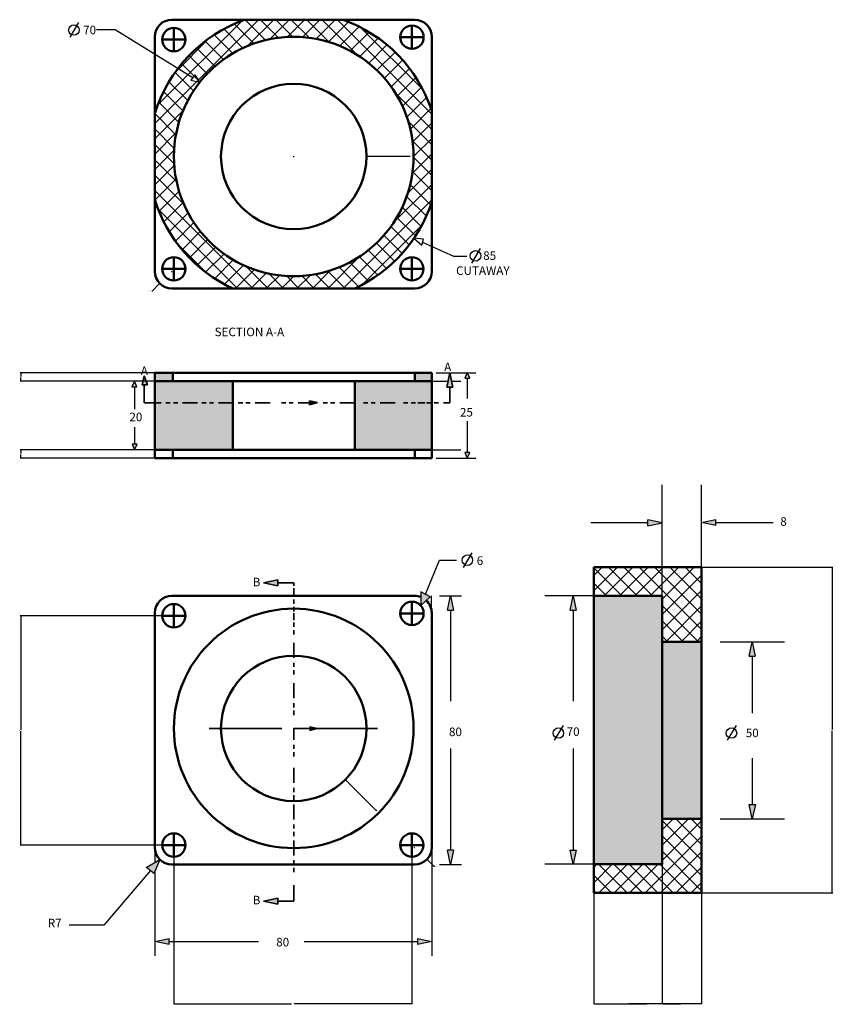
# Model space of a CAD drawing. Units: millimetres. Extents: x 2682 to 5504, y 1503 to 3069.
# Tile 1 of 1: x 2682.4 to 2920.1, y 1503.5 to 1791.3. Entities that reach past the tile are written whole.
import ezdxf

# ---------------------------------------------------------------- set-up
doc = ezdxf.new("R2010")
doc.units = ezdxf.units.MM
doc.linetypes.add('PHANTOM', pattern=[63.5, 31.75, -6.35, 6.35, -6.35, 6.35, -6.35])
for name, color, linetype, lineweight in [('M-DIMS', 2, 'Continuous', 25), ('M-HATC', 8, 'Continuous', 18), ('M-OUTL', 7, 'Continuous', 50), ('M-SECT', 1, 'PHANTOM', 35), ('M-TEXT', 7, 'Continuous', 25)]:
    doc.layers.add(name, color=color, linetype=linetype, lineweight=lineweight)
doc.styles.get("Standard").update_dxf_attribs({"font": 'arial.ttf'})
doc.dimstyles.get("Standard").update_dxf_attribs({"dimtxt": 0.18, "dimasz": 0.18, "dimexe": 0.18, "dimexo": 0.0625, "dimgap": 0.09, "dimtad": 0, "dimtih": 1, "dimtoh": 1, "dimdec": 4, "dimzin": 0, "dimdsep": 46, "dimtxsty": 'Standard', "dimcen": 0.09, "dimadec": 0, "dimazin": 0, "dimtfac": 1, "dimtdec": 4, "dimtofl": 0, "dimtmove": 0, "dimatfit": 3, "dimfxl": 1, "dimtolj": 1, "dimtzin": 0, "dimarcsym": 0})

# ---------------------------------------------------------------- blocks, each defined once
blk = doc.blocks.new('HOLE-6')
for p, q in [((2727.41, 1721.83), (2727.41, 1715)), ((2724, 1718.42), (2730.82, 1718.42))]:
    blk.add_line(p, q)
blk.add_circle((2727.41, 1718.42), 3.41)
blk = doc.blocks.new('*D2')
at = {"layer": 'Defpoints', "color": 0, "transparency": 16777216}
for p in [(2727.41, 1550.02), (2796.97, 1550.02), (2796.97, 1503.64)]:
    blk.add_point(p, dxfattribs=at)
at = {"layer": 'M-DIMS', "color": 0, "lineweight": -2, "transparency": 16777216}
for p, q in [((2727.41, 1549.96), (2727.41, 1503.46)), ((2796.97, 1549.96), (2796.97, 1503.46)), ((2727.59, 1503.64), (2761.79, 1503.64)), ((2796.79, 1503.64), (2762.58, 1503.64))]:
    blk.add_line(p, q, dxfattribs=at)
at = {"layer": 'M-DIMS', "color": 0, "transparency": 16777216}
for points in [[(2727.59, 1503.67), (2727.59, 1503.61), (2727.41, 1503.64)], [(2796.79, 1503.67), (2796.79, 1503.61), (2796.97, 1503.64)]]:
    blk.add_solid(points, dxfattribs=at)
at = {"layer": 'M-DIMS', "color": 0, "transparency": 16777216, "insert": (2762.19, 1503.64), "char_height": 0.18, "attachment_point": 5}
blk.add_mtext('\\A1;69.56', dxfattribs=at)
blk = doc.blocks.new('*D3')
at = {"layer": 'Defpoints', "color": 0, "transparency": 16777216}
for p in [(2682.68, 1617.03), (2727.41, 1617.03), (2727.41, 1550.02)]:
    blk.add_point(p, dxfattribs=at)
at = {"layer": 'M-DIMS', "color": 0, "lineweight": -2, "transparency": 16777216}
for p, q in [((2727.35, 1617.03), (2682.5, 1617.03)), ((2682.68, 1616.85), (2682.68, 1583.71)), ((2682.68, 1550.2), (2682.68, 1583.34)), ((2727.35, 1550.02), (2682.5, 1550.02))]:
    blk.add_line(p, q, dxfattribs=at)
at = {"layer": 'M-DIMS', "color": 0, "transparency": 16777216}
for points in [[(2682.65, 1616.85), (2682.71, 1616.85), (2682.68, 1617.03)], [(2682.65, 1550.2), (2682.71, 1550.2), (2682.68, 1550.02)]]:
    blk.add_solid(points, dxfattribs=at)
at = {"layer": 'M-DIMS', "color": 0, "transparency": 16777216, "insert": (2682.68, 1583.52), "char_height": 0.18, "attachment_point": 5}
blk.add_mtext('\\A1;67.01', dxfattribs=at)
blk = doc.blocks.new('*D4')
at = {"layer": 'Defpoints', "color": 0, "transparency": 16777216}
for p in [(2850.11, 1544.38), (2870.11, 1544.38), (2870.11, 1503.64)]:
    blk.add_point(p, dxfattribs=at)
at = {"layer": 'M-DIMS', "color": 0, "lineweight": -2, "transparency": 16777216}
for p, q in [((2850.11, 1544.32), (2850.11, 1503.46)), ((2870.11, 1544.32), (2870.11, 1503.46)), ((2850.29, 1503.64), (2859.89, 1503.64)), ((2869.93, 1503.64), (2860.33, 1503.64))]:
    blk.add_line(p, q, dxfattribs=at)
at = {"layer": 'M-DIMS', "color": 0, "transparency": 16777216}
for points in [[(2850.29, 1503.67), (2850.29, 1503.61), (2850.11, 1503.64)], [(2869.93, 1503.67), (2869.93, 1503.61), (2870.11, 1503.64)]]:
    blk.add_solid(points, dxfattribs=at)
at = {"layer": 'M-DIMS', "color": 0, "transparency": 16777216, "insert": (2860.11, 1503.64), "char_height": 0.18, "attachment_point": 5}
blk.add_mtext('\\A1;20', dxfattribs=at)
blk = doc.blocks.new('*D5')
at = {"layer": 'Defpoints', "color": 0, "transparency": 16777216}
for p in [(2850.11, 1536.01), (2881.63, 1536.01), (2881.63, 1503.64)]:
    blk.add_point(p, dxfattribs=at)
at = {"layer": 'M-DIMS', "color": 0, "lineweight": -2, "transparency": 16777216}
for p, q in [((2850.11, 1535.95), (2850.11, 1503.46)), ((2881.63, 1535.95), (2881.63, 1503.46)), ((2850.29, 1503.64), (2865.48, 1503.64)), ((2881.45, 1503.64), (2866.26, 1503.64))]:
    blk.add_line(p, q, dxfattribs=at)
at = {"layer": 'M-DIMS', "color": 0, "transparency": 16777216}
for points in [[(2850.29, 1503.67), (2850.29, 1503.61), (2850.11, 1503.64)], [(2881.45, 1503.67), (2881.45, 1503.61), (2881.63, 1503.64)]]:
    blk.add_solid(points, dxfattribs=at)
at = {"layer": 'M-DIMS', "color": 0, "transparency": 16777216, "insert": (2865.87, 1503.64), "char_height": 0.18, "attachment_point": 5}
blk.add_mtext('\\A1;31.52', dxfattribs=at)
blk = doc.blocks.new('*D6')
at = {"layer": 'Defpoints', "color": 0, "transparency": 16777216}
for p in [(2881.63, 1631.23), (2919.79, 1631.23), (2881.63, 1536.01)]:
    blk.add_point(p, dxfattribs=at)
at = {"layer": 'M-DIMS', "color": 0, "lineweight": -2, "transparency": 16777216}
for p, q in [((2881.69, 1631.23), (2919.97, 1631.23)), ((2919.79, 1631.05), (2919.79, 1583.8)), ((2919.79, 1536.19), (2919.79, 1583.44)), ((2881.69, 1536.01), (2919.97, 1536.01))]:
    blk.add_line(p, q, dxfattribs=at)
at = {"layer": 'M-DIMS', "color": 0, "transparency": 16777216}
for points in [[(2919.76, 1631.05), (2919.82, 1631.05), (2919.79, 1631.23)], [(2919.76, 1536.19), (2919.82, 1536.19), (2919.79, 1536.01)]]:
    blk.add_solid(points, dxfattribs=at)
at = {"layer": 'M-DIMS', "color": 0, "transparency": 16777216, "insert": (2919.79, 1583.62), "char_height": 0.18, "attachment_point": 5}
blk.add_mtext('\\A1;95.22', dxfattribs=at)
blk = doc.blocks.new('*D7')
at = {"layer": 'Defpoints', "color": 0, "transparency": 16777216}
for p in [(2721.84, 1688.06), (2682.68, 1685.56), (2721.84, 1685.56)]:
    blk.add_point(p, dxfattribs=at)
at = {"layer": 'M-DIMS', "color": 0, "lineweight": -2, "transparency": 16777216}
for p, q in [((2721.77, 1688.06), (2682.5, 1688.06)), ((2682.68, 1687.88), (2682.68, 1686.99)), ((2682.68, 1685.74), (2682.68, 1686.63)), ((2721.77, 1685.56), (2682.5, 1685.56))]:
    blk.add_line(p, q, dxfattribs=at)
at = {"layer": 'M-DIMS', "color": 0, "transparency": 16777216}
for points in [[(2682.65, 1687.88), (2682.71, 1687.88), (2682.68, 1688.06)], [(2682.65, 1685.74), (2682.71, 1685.74), (2682.68, 1685.56)]]:
    blk.add_solid(points, dxfattribs=at)
at = {"layer": 'M-DIMS', "color": 0, "transparency": 16777216, "insert": (2682.68, 1686.81), "char_height": 0.18, "attachment_point": 5}
blk.add_mtext('\\A1;2.5', dxfattribs=at)
blk = doc.blocks.new('*D8')
at = {"layer": 'Defpoints', "color": 0, "transparency": 16777216}
for p in [(2747.38, 1599.11), (2777.49, 1569.11)]:
    blk.add_point(p, dxfattribs=at)
at = {"layer": 'M-DIMS', "color": 0, "lineweight": -2, "transparency": 16777216}
for p, q in [((2762.35, 1584.11), (2762.53, 1584.11)), ((2762.44, 1584.02), (2762.44, 1584.2)), ((2786.52, 1560.11), (2777.62, 1568.98)), ((2786.7, 1560.11), (2786.52, 1560.11))]:
    blk.add_line(p, q, dxfattribs=at)
at = {"layer": 'M-DIMS', "color": 0, "transparency": 16777216}
blk.add_solid([(2777.64, 1569), (2777.6, 1568.96), (2777.49, 1569.11)], dxfattribs=at)
at = {"layer": 'M-DIMS', "color": 0, "transparency": 16777216, "insert": (2787.12, 1560.11), "char_height": 0.18, "attachment_point": 5}
blk.add_mtext('\\A1;∅42.5', dxfattribs=at)
blk = doc.blocks.new('*D9')
at = {"layer": 'Defpoints', "color": 0, "transparency": 16777216}
for p in [(2881.63, 1631.23), (2870.11, 1609.4), (2881.63, 1503.64)]:
    blk.add_point(p, dxfattribs=at)
at = {"layer": 'M-DIMS', "color": 0, "lineweight": -2, "transparency": 16777216}
for p, q in [((2881.63, 1631.17), (2881.63, 1503.46)), ((2870.11, 1609.34), (2870.11, 1503.46)), ((2870.29, 1503.64), (2875.49, 1503.64)), ((2881.45, 1503.64), (2876.25, 1503.64))]:
    blk.add_line(p, q, dxfattribs=at)
at = {"layer": 'M-DIMS', "color": 0, "transparency": 16777216}
for points in [[(2870.29, 1503.67), (2870.29, 1503.61), (2870.11, 1503.64)], [(2881.45, 1503.67), (2881.45, 1503.61), (2881.63, 1503.64)]]:
    blk.add_solid(points, dxfattribs=at)
at = {"layer": 'M-DIMS', "color": 0, "transparency": 16777216, "insert": (2875.87, 1503.64), "char_height": 0.18, "attachment_point": 5}
blk.add_mtext('\\A1;11.52', dxfattribs=at)
blk = doc.blocks.new('*D10')
at = {"layer": 'Defpoints', "color": 0, "transparency": 16777216}
for p in [(2721.84, 1665.56), (2682.68, 1663.06), (2721.84, 1663.06)]:
    blk.add_point(p, dxfattribs=at)
at = {"layer": 'M-DIMS', "color": 0, "lineweight": -2, "transparency": 16777216}
for p, q in [((2721.77, 1665.56), (2682.5, 1665.56)), ((2682.68, 1665.38), (2682.68, 1664.49)), ((2682.68, 1663.24), (2682.68, 1664.13)), ((2721.77, 1663.06), (2682.5, 1663.06))]:
    blk.add_line(p, q, dxfattribs=at)
at = {"layer": 'M-DIMS', "color": 0, "transparency": 16777216}
for points in [[(2682.65, 1665.38), (2682.71, 1665.38), (2682.68, 1665.56)], [(2682.65, 1663.24), (2682.71, 1663.24), (2682.68, 1663.06)]]:
    blk.add_solid(points, dxfattribs=at)
at = {"layer": 'M-DIMS', "color": 0, "transparency": 16777216, "insert": (2682.68, 1664.31), "char_height": 0.18, "attachment_point": 5}
blk.add_mtext('\\A1;2.50', dxfattribs=at)
blk = doc.blocks.new('*D11')
at = {"layer": 'Defpoints', "color": 0, "transparency": 16777216}
for p in [(2726.84, 1717.7), (2723.3, 1714.16)]:
    blk.add_point(p, dxfattribs=at)
at = {"layer": 'M-DIMS', "color": 0, "lineweight": -2, "transparency": 16777216}
for p, q in [((2726.75, 1717.7), (2726.93, 1717.7)), ((2726.84, 1717.61), (2726.84, 1717.79)), ((2721.18, 1712.04), (2723.17, 1714.04)), ((2721, 1712.04), (2721.18, 1712.04))]:
    blk.add_line(p, q, dxfattribs=at)
at = {"layer": 'M-DIMS', "color": 0, "transparency": 16777216}
blk.add_solid([(2723.15, 1714.06), (2723.19, 1714.01), (2723.3, 1714.16)], dxfattribs=at)
at = {"layer": 'M-DIMS', "color": 0, "transparency": 16777216, "insert": (2720.39, 1712.04), "char_height": 0.18, "attachment_point": 5}
blk.add_mtext('\\A1;4X R5.00', dxfattribs=at)
blk = doc.blocks.new('*D12')
at = {"layer": 'Defpoints', "color": 0, "transparency": 16777216}
for p in [(2797.77, 1549.3), (2801.36, 1545.82)]:
    blk.add_point(p, dxfattribs=at)
at = {"layer": 'M-DIMS', "color": 0, "lineweight": -2, "transparency": 16777216}
for p, q in [((2797.68, 1549.3), (2797.86, 1549.3)), ((2797.77, 1549.21), (2797.77, 1549.39)), ((2803.52, 1543.73), (2801.49, 1545.7)), ((2803.7, 1543.73), (2803.52, 1543.73))]:
    blk.add_line(p, q, dxfattribs=at)
at = {"layer": 'M-DIMS', "color": 0, "transparency": 16777216}
blk.add_solid([(2801.52, 1545.72), (2801.47, 1545.67), (2801.36, 1545.82)], dxfattribs=at)
at = {"layer": 'M-DIMS', "color": 0, "transparency": 16777216, "insert": (2804.31, 1543.73), "char_height": 0.18, "attachment_point": 5}
blk.add_mtext('\\A1;4X R5.00', dxfattribs=at)
blk = doc.blocks.new('*D13')
at = {"layer": 'Defpoints', "color": 0, "transparency": 16777216}
for p in [(2741.19, 1751.28), (2783.69, 1751.28)]:
    blk.add_point(p, dxfattribs=at)
at = {"layer": 'M-DIMS', "color": 0, "lineweight": -2, "transparency": 16777216}
for p, q in [((2762.35, 1751.28), (2762.53, 1751.28)), ((2762.44, 1751.19), (2762.44, 1751.37)), ((2796.44, 1751.28), (2783.87, 1751.28))]:
    blk.add_line(p, q, dxfattribs=at)
at = {"layer": 'M-DIMS', "color": 0, "transparency": 16777216}
blk.add_solid([(2783.87, 1751.31), (2783.87, 1751.25), (2783.69, 1751.28)], dxfattribs=at)
at = {"layer": 'M-DIMS', "color": 0, "transparency": 16777216, "insert": (2796.93, 1751.28), "char_height": 0.18, "attachment_point": 5}
blk.add_mtext('\\A1;∅42.50', dxfattribs=at)

msp = doc.modelspace()

# ---------------------------------------------------------------- hatches: boundary and pattern name
at = {"layer": 'M-DIMS'}
h = msp.add_hatch(color=256, dxfattribs=at)
h.dxf.hatch_style = 1
h.paths.add_polyline_path([(2715.954, 1685.563), (2715.185, 1683.9), (2716.643, 1683.9)])
h.paths.add_polyline_path([(2718.77, 1687.184), (2718.139, 1684.573), (2719.674, 1684.573)])
h.paths.add_polyline_path([(2716.723, 1667.225), (2715.264, 1667.225), (2715.954, 1665.563)])
h.paths.add_polyline_path([(2813.896, 1664.741), (2812.437, 1664.741), (2813.127, 1663.078)])
h.paths.add_polyline_path([(2813.184, 1688.063), (2813.148, 1688.063), (2812.398, 1686.441), (2813.857, 1686.441)])
h.paths.add_polyline_path([(2808.083, 1688.063), (2807.195, 1683.887), (2808.962, 1683.887)])
h = msp.add_hatch(color=256, dxfattribs=at)
h.dxf.hatch_style = 1
h.paths.add_polyline_path([(2865.934, 1645.043), (2865.934, 1643.277), (2870.11, 1644.165)])
h.paths.add_polyline_path([(2885.806, 1645.132), (2881.63, 1644.253), (2885.806, 1643.365)])
h.paths.add_polyline_path([(2844.062, 1622.82), (2843.174, 1618.644), (2844.94, 1618.644)])
h.paths.add_polyline_path([(2896.438, 1609.402), (2895.55, 1605.226), (2897.316, 1605.226)])
h.paths.add_polyline_path([(2844.95, 1548.557), (2843.184, 1548.557), (2844.062, 1544.381)])
h.paths.add_polyline_path([(2897.326, 1561.875), (2895.56, 1561.875), (2896.438, 1557.699)])
h = msp.add_hatch(color=256, dxfattribs=at)
h.dxf.hatch_style = 1
h.paths.add_polyline_path([(2757.796, 1534.519), (2753.62, 1533.641), (2757.796, 1532.753)])
h.paths.add_polyline_path([(2757.796, 1627.506), (2753.62, 1626.628), (2757.796, 1625.74)])
h = msp.add_hatch(color=256, dxfattribs=at)
h.dxf.hatch_style = 1
h.paths.add_polyline_path([(2799.554, 1624.01), (2799.554, 1620.003, -0.0017904), (2799.57, 1619.984), (2802.295, 1622.604)])
h = msp.add_hatch(color=256, dxfattribs=at)
h.dxf.hatch_style = 1
h.paths.add_polyline_path([(2808.251, 1622.82), (2807.363, 1618.644), (2809.129, 1618.644)])
h.paths.add_polyline_path([(2809.139, 1548.474), (2807.373, 1548.474), (2808.251, 1544.298)])
h.paths.add_polyline_path([(2802.772, 1521.845), (2798.596, 1522.733), (2798.596, 1520.967)])
h.paths.add_polyline_path([(2726.014, 1522.719), (2721.837, 1521.845), (2726.012, 1520.952)])
h.paths.add_polyline_path([(2723.301, 1545.762), (2719.332, 1543.416), (2720.212, 1542.815), (2721.671, 1541.819)])
at = {"layer": 'M-HATC'}
h = msp.add_hatch(dxfattribs=at)
h.set_pattern_fill('ANSI37', color=256)
h.paths.add_polyline_path([(2776.856, 1791.259), (2748.017, 1791.259, 0.2353251), (2721.837, 1763.846), (2721.837, 1738.714, 0.212581), (2744.612, 1712.698), (2780.261, 1712.698, 0.2072631), (2802.772, 1737.889), (2802.772, 1764.671, 0.229956)])
h.paths.add_polyline_path([(2797.436, 1751.28, -1), (2727.436, 1751.28, -1)], flags=16)
h.paths.add_polyline_path([(2783.686, 1751.28, -1), (2741.186, 1751.28, -1)], flags=0)
h = msp.add_hatch(color=256, dxfattribs=at)
h.dxf.hatch_style = 1
h.set_gradient(color1=(69, 84, 165))
h.paths.add_polyline_path([(2727.092, 1688.063), (2721.837, 1688.063), (2721.837, 1685.563), (2727.092, 1685.563)])
h = msp.add_hatch(color=256, dxfattribs=at)
h.dxf.hatch_style = 1
h.set_gradient(color1=(255, 255, 255), color2=(69, 84, 165))
h.paths.add_polyline_path([(2802.772, 1688.063), (2797.847, 1688.063), (2797.847, 1685.563), (2802.772, 1685.563)])
h.paths.add_polyline_path([(2802.772, 1685.563), (2797.847, 1685.563), (2780.261, 1685.563), (2780.261, 1665.563), (2802.772, 1665.563)])
h = msp.add_hatch(color=256, dxfattribs=at)
h.dxf.hatch_style = 1
h.set_gradient(color1=(69, 84, 165))
h.paths.add_polyline_path([(2744.612, 1685.563), (2721.837, 1685.563), (2721.837, 1665.563), (2744.612, 1665.563)])
h = msp.add_hatch(dxfattribs=at)
h.set_pattern_fill('ANSI37', color=256)
h.paths.add_polyline_path([(2881.63, 1631.232), (2850.11, 1631.232), (2850.11, 1622.859), (2870.11, 1622.859), (2870.11, 1609.402), (2881.63, 1609.402)])
h.paths.add_polyline_path([(2881.63, 1557.699), (2870.11, 1557.699), (2870.11, 1544.381), (2850.11, 1544.381), (2850.11, 1536.011), (2881.63, 1536.011)])
h = msp.add_hatch(color=256, dxfattribs=at)
h.dxf.hatch_style = 1
h.set_gradient(color1=(69, 84, 165))
h.paths.add_polyline_path([(2870.11, 1544.381), (2870.11, 1622.859), (2850.11, 1622.859), (2850.11, 1544.381)])
h.paths.add_polyline_path([(2881.63, 1557.699), (2881.63, 1609.402), (2870.11, 1609.402), (2870.11, 1557.699)])
at = {"layer": 'M-SECT'}
h = msp.add_hatch(color=256, dxfattribs=at)
h.dxf.hatch_style = 1
h.paths.add_polyline_path([(2769.415, 1679.384), (2767.094, 1679.869), (2767.094, 1678.731)])
h = msp.add_hatch(color=256, dxfattribs=at)
h.dxf.hatch_style = 1
h.paths.add_polyline_path([(2769.415, 1584.104), (2767.094, 1584.589), (2767.094, 1583.451)])

# ---------------------------------------------------------------- linework, layer by layer
at = {"layer": 'M-DIMS'}
for p, q in [((2699.559, 1790.403), (2696.997, 1786.118)), ((2710.286, 1788.25), (2704.783, 1788.25)), ((2732.939, 1774.293), (2710.286, 1788.25)), ((2733.619, 1775.152), (2732.38, 1773.587)), ((2732.38, 1773.587), (2735.006, 1773.019)), ((2735.006, 1773.019), (2733.619, 1775.152)), ((2797.567, 1727.361), (2799.86, 1725.306)), ((2800.365, 1727.13), (2797.567, 1727.361)), ((2799.86, 1725.306), (2800.365, 1727.13)), ((2800.111, 1726.211), (2809.089, 1722.152)), ((2816.899, 1724.402), (2814.337, 1720.116)), ((2809.089, 1722.152), (2813.032, 1722.152)), ((2804.1, 1688.063), (2815.663, 1688.063)), ((2813.167, 1688.104), (2812.398, 1686.441)), ((2813.857, 1686.441), (2813.167, 1688.104)), ((2718.378, 1685.563), (2710.071, 1685.563)), ((2715.954, 1685.563), (2715.185, 1683.9)), ((2715.185, 1683.9), (2716.643, 1683.9)), ((2716.643, 1683.9), (2715.954, 1685.563)), ((2715.954, 1683.9), (2715.954, 1677.378)), ((2721.837, 1685.563), (2719.331, 1685.563)), ((2802.772, 1685.563), (2807.552, 1685.563)), ((2808.609, 1685.563), (2811.272, 1685.563)), ((2812.398, 1686.441), (2813.857, 1686.441)), ((2813.167, 1686.441), (2813.167, 1680.511)), ((2715.954, 1672.162), (2715.954, 1667.225)), ((2813.167, 1673.937), (2813.167, 1664.741)), ((2716.723, 1667.225), (2715.264, 1667.225)), ((2715.264, 1667.225), (2715.954, 1665.563)), ((2715.954, 1665.563), (2716.723, 1667.225)), ((2721.837, 1665.563), (2710.071, 1665.563)), ((2802.772, 1665.563), (2811.272, 1665.563)), ((2813.896, 1664.741), (2812.437, 1664.741)), ((2812.437, 1664.741), (2813.127, 1663.078)), ((2813.127, 1663.078), (2813.896, 1664.741)), ((2804.1, 1663.063), (2815.663, 1663.063)), ((2813.167, 1663.164), (2813.167, 1663.063)), ((2870.11, 1622.859), (2870.11, 1655.326)), ((2881.63, 1631.232), (2881.63, 1655.326)), ((2865.934, 1644.165), (2849.244, 1644.165)), ((2865.934, 1643.277), (2865.934, 1645.043)), ((2870.11, 1644.165), (2865.934, 1645.043)), ((2865.934, 1643.277), (2865.934, 1645.043)), ((2870.11, 1644.165), (2865.934, 1645.043)), ((2865.934, 1643.277), (2870.11, 1644.165)), ((2865.934, 1643.277), (2870.11, 1644.165)), ((2881.63, 1644.253), (2885.806, 1645.132)), ((2881.63, 1644.253), (2885.806, 1645.132)), ((2885.806, 1643.365), (2881.63, 1644.253)), ((2885.806, 1643.365), (2881.63, 1644.253)), ((2885.806, 1643.365), (2885.806, 1645.132)), ((2885.806, 1643.365), (2885.806, 1645.132)), ((2885.806, 1644.253), (2902.496, 1644.253)), ((2814.529, 1635.453), (2811.967, 1631.167)), ((2800.934, 1623.302), (2805.048, 1633.31)), ((2805.048, 1633.31), (2810.002, 1633.31)), ((2802.295, 1622.604), (2799.554, 1624.01)), ((2799.554, 1624.01), (2799.554, 1620.003)), ((2799.57, 1619.984), (2802.295, 1622.604)), ((2802.666, 1618.881), (2802.666, 1622.82)), ((2805.048, 1622.82), (2811.453, 1622.82)), ((2807.363, 1618.644), (2808.251, 1622.82)), ((2808.251, 1622.82), (2809.129, 1618.644)), ((2850.11, 1622.859), (2835.789, 1622.859)), ((2835.789, 1622.859), (2835.789, 1622.859)), ((2843.174, 1618.644), (2844.062, 1622.82)), ((2844.062, 1622.82), (2844.94, 1618.644)), ((2807.363, 1618.644), (2809.129, 1618.644)), ((2808.251, 1618.644), (2808.251, 1592.071)), ((2843.174, 1618.644), (2844.94, 1618.644)), ((2844.062, 1618.644), (2844.062, 1592.071)), ((2887.083, 1609.402), (2905.793, 1609.402)), ((2895.55, 1605.226), (2896.438, 1609.402)), ((2895.55, 1605.226), (2896.438, 1609.402)), ((2896.438, 1609.402), (2897.316, 1605.226)), ((2896.438, 1609.402), (2897.316, 1605.226)), ((2895.55, 1605.226), (2897.316, 1605.226)), ((2895.55, 1605.226), (2897.316, 1605.226)), ((2896.438, 1605.226), (2896.438, 1588.536)), ((2841.122, 1584.915), (2838.559, 1580.63)), ((2891.685, 1584.915), (2889.123, 1580.63)), ((2808.251, 1578.22), (2808.251, 1548.474)), ((2844.062, 1578.22), (2844.062, 1548.557)), ((2896.438, 1575.406), (2896.438, 1561.875)), ((2896.438, 1557.699), (2895.56, 1561.875)), ((2895.56, 1561.875), (2897.326, 1561.875)), ((2897.326, 1561.875), (2896.438, 1557.699)), ((2887.083, 1557.699), (2905.793, 1557.699)), ((2721.837, 1549.298), (2721.837, 1544.897)), ((2802.772, 1549.298), (2802.772, 1517.637)), ((2809.139, 1548.474), (2807.373, 1548.474)), ((2808.251, 1544.298), (2807.373, 1548.474)), ((2809.139, 1548.474), (2808.251, 1544.298)), ((2844.062, 1544.381), (2843.184, 1548.557)), ((2843.184, 1548.557), (2844.95, 1548.557)), ((2844.95, 1548.557), (2844.062, 1544.381)), ((2719.332, 1543.416), (2723.301, 1545.762)), ((2723.301, 1545.762), (2721.671, 1541.819)), ((2720.212, 1542.815), (2719.332, 1543.416)), ((2720.212, 1542.815), (2721.671, 1541.819)), ((2805.048, 1544.298), (2811.453, 1544.298)), ((2850.11, 1544.381), (2835.789, 1544.381)), ((2720.579, 1542.564), (2706.963, 1526.564)), ((2721.837, 1542.221), (2721.837, 1517.637)), ((2706.963, 1526.564), (2696.837, 1526.564)), ((2721.837, 1521.845), (2726.014, 1522.719)), ((2726.012, 1520.952), (2726.014, 1522.719)), ((2798.596, 1522.733), (2798.596, 1520.967)), ((2798.596, 1522.733), (2802.772, 1521.845)), ((2726.012, 1520.952), (2721.837, 1521.845)), ((2726.013, 1521.845), (2752.192, 1521.845)), ((2765.468, 1521.845), (2798.596, 1521.845)), ((2802.772, 1521.845), (2798.596, 1520.967))]:
    msp.add_line(p, q, dxfattribs=at)
for centre in [(2698.214, 1788.229), (2815.554, 1722.227), (2813.184, 1633.278), (2839.776, 1582.741), (2890.34, 1582.741)]:
    msp.add_circle(centre, 1.535, dxfattribs=at)
at = {"layer": 'M-OUTL'}
for p, q in [((2744.612, 1791.259), (2726.837, 1791.259)), ((2744.612, 1791.259), (2797.772, 1791.259)), ((2721.837, 1763.846), (2721.837, 1786.259)), ((2802.772, 1764.671), (2802.772, 1786.259)), ((2802.772, 1764.671), (2802.772, 1717.698)), ((2721.837, 1763.846), (2721.837, 1738.714)), ((2721.837, 1738.714), (2721.837, 1717.698)), ((2723.995, 1718.418), (2723.995, 1718.418)), ((2744.612, 1712.698), (2726.837, 1712.698)), ((2744.612, 1712.698), (2797.772, 1712.698)), ((2721.837, 1688.063), (2721.837, 1663.063)), ((2802.772, 1688.063), (2721.837, 1688.063)), ((2727.092, 1688.063), (2727.092, 1685.563)), ((2797.847, 1688.063), (2797.847, 1685.563)), ((2802.772, 1663.063), (2802.772, 1688.063)), ((2721.837, 1685.563), (2802.772, 1685.563)), ((2744.612, 1685.563), (2744.612, 1665.563)), ((2780.261, 1685.563), (2780.261, 1665.563)), ((2802.772, 1665.563), (2721.837, 1665.563)), ((2727.092, 1665.563), (2727.092, 1663.063)), ((2797.847, 1665.563), (2797.847, 1663.063)), ((2721.837, 1663.063), (2802.772, 1663.063)), ((2850.11, 1622.859), (2850.11, 1631.232)), ((2850.11, 1631.232), (2881.63, 1631.232)), ((2881.63, 1631.232), (2881.63, 1609.402)), ((2744.612, 1622.859), (2726.837, 1622.859)), ((2744.612, 1622.859), (2797.772, 1622.859)), ((2850.11, 1622.859), (2870.11, 1622.859)), ((2850.11, 1622.859), (2850.11, 1544.381)), ((2870.11, 1544.381), (2870.11, 1622.859)), ((2721.837, 1549.298), (2721.837, 1617.859)), ((2802.772, 1596.27), (2802.772, 1617.859)), ((2870.11, 1609.402), (2881.63, 1609.402)), ((2881.63, 1609.402), (2881.63, 1557.699)), ((2802.772, 1596.27), (2802.772, 1549.298)), ((2721.837, 1570.313), (2721.837, 1549.298)), ((2881.63, 1557.699), (2870.11, 1557.699)), ((2881.63, 1536.011), (2881.63, 1557.699)), ((2744.612, 1544.298), (2726.837, 1544.298)), ((2744.612, 1544.298), (2797.772, 1544.298)), ((2850.11, 1544.381), (2870.11, 1544.381)), ((2850.11, 1544.381), (2850.11, 1536.011)), ((2850.11, 1536.011), (2881.63, 1536.011))]:
    msp.add_line(p, q, dxfattribs=at)
for centre, radius in [((2762.436, 1751.28), 35), ((2762.436, 1751.28), 21.25), ((2762.436, 1584.11), 35), ((2762.436, 1584.11), 21.25)]:
    msp.add_circle(centre, radius, dxfattribs=at)
for centre, radius, start, end in [((2762.436, 1751.28), 42.5, 109.83308, 162.8019), ((2726.837, 1786.259), 5, 90, 180), ((2762.436, 1751.28), 42.5, 18.36544, 70.16692), ((2797.772, 1786.259), 5, 0, 90), ((2762.436, 1751.28), 42.5, 197.1981, 245.20347), ((2762.436, 1751.28), 42.5, 294.79653, 341.63456), ((2726.837, 1717.698), 5, 180, 270), ((2797.772, 1717.698), 5, 270, 0), ((2726.837, 1617.859), 5, 90, 180), ((2797.772, 1617.859), 5, 69.11832, 90), ((2797.772, 1617.859), 5, 0, 47.15199), ((2726.837, 1549.298), 5, 180, 270), ((2797.772, 1549.298), 5, 270, 0)]:
    msp.add_arc(centre, radius, start, end, dxfattribs=at)
at = {"layer": 'M-SECT'}
for p, q in [((2718.77, 1687.184), (2718.139, 1684.573)), ((2719.674, 1684.573), (2718.77, 1687.184)), ((2807.195, 1683.887), (2808.083, 1688.063)), ((2808.083, 1688.063), (2808.083, 1688.063)), ((2808.083, 1688.063), (2808.962, 1683.887)), ((2718.139, 1684.573), (2719.674, 1684.573)), ((2718.77, 1684.573), (2718.77, 1679.247)), ((2807.195, 1683.887), (2808.962, 1683.887)), ((2808.078, 1679.247), (2808.078, 1683.887)), ((2718.77, 1679.247), (2723.715, 1679.247)), ((2725.073, 1679.247), (2726.364, 1679.247)), ((2727.298, 1679.247), (2728.533, 1679.247)), ((2729.961, 1679.247), (2734.355, 1679.247)), ((2735.563, 1679.247), (2736.854, 1679.247)), ((2737.788, 1679.247), (2739.023, 1679.247)), ((2740.451, 1679.247), (2744.845, 1679.247)), ((2746.247, 1679.247), (2747.538, 1679.247)), ((2748.471, 1679.247), (2749.707, 1679.247)), ((2751.135, 1679.247), (2755.529, 1679.247)), ((2758.86, 1679.247), (2760.15, 1679.247)), ((2761.084, 1679.247), (2762.32, 1679.247)), ((2763.748, 1679.247), (2767.094, 1679.247)), ((2767.094, 1679.869), (2767.094, 1678.731)), ((2769.415, 1679.384), (2767.094, 1679.869)), ((2767.094, 1678.731), (2769.415, 1679.384)), ((2771, 1679.247), (2772.29, 1679.247)), ((2773.224, 1679.247), (2774.46, 1679.247)), ((2775.888, 1679.247), (2780.281, 1679.247)), ((2782.812, 1679.247), (2784.103, 1679.247)), ((2785.036, 1679.247), (2786.272, 1679.247)), ((2787.7, 1679.247), (2792.094, 1679.247)), ((2794.535, 1679.247), (2795.826, 1679.247)), ((2796.76, 1679.247), (2797.995, 1679.247)), ((2798.689, 1679.247), (2800.771, 1679.247)), ((2801.283, 1679.247), (2802.574, 1679.247)), ((2803.508, 1679.247), (2804.743, 1679.247)), ((2806.173, 1679.247), (2808.078, 1679.247)), ((2753.62, 1626.628), (2757.796, 1627.506)), ((2757.796, 1625.74), (2753.62, 1626.628)), ((2757.796, 1625.74), (2757.796, 1627.506)), ((2762.436, 1626.623), (2757.796, 1626.623)), ((2762.436, 1626.623), (2762.436, 1625.78)), ((2762.436, 1623.189), (2762.436, 1625.094)), ((2762.436, 1620.523), (2762.436, 1621.759)), ((2762.436, 1618.299), (2762.436, 1619.59)), ((2762.436, 1615.705), (2762.436, 1617.787)), ((2762.436, 1613.775), (2762.436, 1615.011)), ((2762.436, 1611.551), (2762.436, 1612.842)), ((2762.436, 1604.716), (2762.436, 1609.11)), ((2762.436, 1602.052), (2762.436, 1603.288)), ((2762.436, 1599.828), (2762.436, 1601.119)), ((2762.436, 1592.903), (2762.436, 1597.297)), ((2762.436, 1590.24), (2762.436, 1591.475)), ((2762.436, 1588.015), (2762.436, 1589.306)), ((2755.614, 1584.11), (2737.701, 1584.11)), ((2755.614, 1584.11), (2758.924, 1584.11)), ((2762.436, 1580.763), (2762.436, 1584.11)), ((2762.436, 1584.11), (2786.961, 1584.11)), ((2769.415, 1584.104), (2767.094, 1584.589)), ((2767.094, 1583.451), (2769.415, 1584.104)), ((2762.436, 1578.1), (2762.436, 1579.335)), ((2762.436, 1575.875), (2762.436, 1577.166)), ((2762.436, 1568.151), (2762.436, 1572.545)), ((2762.436, 1565.487), (2762.436, 1566.723)), ((2762.436, 1563.263), (2762.436, 1564.553)), ((2762.436, 1557.467), (2762.436, 1561.861)), ((2762.436, 1554.803), (2762.436, 1556.039)), ((2762.436, 1552.579), (2762.436, 1553.87)), ((2762.436, 1546.977), (2762.436, 1551.371)), ((2762.436, 1544.313), (2762.436, 1545.549)), ((2762.436, 1542.089), (2762.436, 1543.38)), ((2762.436, 1533.636), (2762.436, 1538.258)), ((2753.62, 1533.641), (2757.796, 1534.519)), ((2757.796, 1532.753), (2757.796, 1534.519)), ((2757.796, 1532.753), (2753.62, 1533.641)), ((2762.436, 1533.636), (2757.796, 1533.636))]:
    msp.add_line(p, q, dxfattribs=at)

# ---------------------------------------------------------------- block references
at = {"layer": 'M-OUTL'}
for p, rotation in [((4445.827, -941.977), 90), ((4515.417, -941.272), 90), ((4445.827, -1008.992), 89.99999999999618), ((4515.384, -1008.992), 89.99999999999618), ((4445.827, -1110.377), 89.99999999998474), ((4515.417, -1109.672), 90), ((4445.827, -1177.392), 89.99999999999618), ((4515.384, -1177.392), 89.99999999999618)]:
    msp.add_blockref('HOLE-6', p, dxfattribs=dict(at, rotation=rotation))

# ---------------------------------------------------------------- texts
at = {"layer": 'M-TEXT', "char_height": 2.5, "attachment_point": 1}
for s, width, insert in [('70', 3.11967, (2700.909, 1789.5)), ('85', 7.61666, (2817.801, 1723.543)), ('CUTAWAY', 11.15524, (2809.884, 1719.157)), ('SECTION A-A', 37.91004, (2739.313, 1701.248)), ('A', 4.12065, (2717.742, 1689.908)), ('A', 4.12065, (2806.406, 1691.027)), ('20', 9.25069, (2714.424, 1676.4)), ('25', 17.23717, (2811.012, 1677.762)), ('8', 19.777, (2904.605, 1645.82)), ('6', 2.5, (2815.913, 1634.397)), ('B', 3.31218, (2750.457, 1628.138)), ('80', 11.8065, (2807.8, 1584.351)), ('70', 7.58221, (2842.187, 1584.401)), ('50', 19.25784, (2894.527, 1584.036)), ('B', 3.31218, (2750.457, 1535.171)), ('R7', 8.78459, (2690.573, 1528.463)), ('80', 11.8065, (2757.326, 1522.88))]:
    msp.add_mtext_dynamic_manual_height_columns(s, width=width, gutter_width=12.5, heights=[0], dxfattribs=dict(at, insert=insert))

# ---------------------------------------------------------------- dimensions: what is measured, and where the dimension line sits
at = {"layer": 'M-DIMS'}
for p1, p2, override, picture, middle in [((2741.186, 1751.28), (2783.686, 1751.28), {"dimdec": 2, "dimlfac": 1, "dimrnd": 0, "dimzin": 0, "dimdsep": 46, "dimlunit": 2}, '*D13', (2796.436, 1751.28)), ((2747.383, 1599.109), (2777.489, 1569.111), {"dimdec": 1, "dimlfac": 1, "dimrnd": 0, "dimzin": 0, "dimdsep": 46, "dimlunit": 2}, '*D8', (2787.124, 1560.111))]:
    dim = msp.add_diameter_dim_2p(p1=p1, p2=p2, dimstyle='Standard', override=override, dxfattribs=at)
    dim.commit()
    dim.dimension.update_dxf_attribs({"geometry": picture, "text_midpoint": middle, "dimtype": 163})
for center, mpoint, picture, middle in [((2726.837, 1717.698), (2723.301, 1714.163), '*D11', (2720.393, 1712.042)), ((2797.772, 1549.298), (2801.365, 1545.821), '*D12', (2804.307, 1543.735))]:
    dim = msp.add_radius_dim(center=center, mpoint=mpoint, text='4X <>', dimstyle='Standard', override={"dimdec": 2, "dimlfac": 1, "dimrnd": 0, "dimzin": 0, "dimdsep": 46, "dimlunit": 2}, dxfattribs=at)
    dim.commit()
    dim.dimension.update_dxf_attribs({"geometry": picture, "text_midpoint": middle, "dimtype": 164})
for base, p1, p2, override, picture, middle in [((2682.679, 1685.563), (2721.837, 1688.063), (2721.837, 1685.563), {"dimdec": 1, "dimlfac": 1, "dimrnd": 0, "dimzin": 0, "dimdsep": 46, "dimlunit": 2}, '*D7', (2682.679, 1686.813)), ((2682.679, 1663.063), (2721.837, 1665.563), (2721.837, 1663.063), {"dimdec": 2, "dimlfac": 1, "dimrnd": 0, "dimzin": 0, "dimdsep": 46, "dimlunit": 2}, '*D10', (2682.679, 1664.313)), ((2919.793, 1631.232), (2881.63, 1536.011), (2881.63, 1631.232), {"dimdec": 2, "dimlfac": 1, "dimrnd": 0, "dimzin": 0, "dimdsep": 46, "dimlunit": 2}, '*D6', (2919.793, 1583.621)), ((2682.679, 1617.032), (2727.409, 1550.018), (2727.409, 1617.032), {"dimdec": 2, "dimlfac": 1, "dimrnd": 0, "dimzin": 0, "dimdsep": 46, "dimlunit": 2}, '*D3', (2682.679, 1583.525))]:
    dim = msp.add_linear_dim(base=base, p1=p1, p2=p2, angle=90, dimstyle='Standard', override=override, dxfattribs=at)
    dim.commit()
    dim.dimension.update_dxf_attribs({"geometry": picture, "text_midpoint": middle})
for base, p1, p2, override, picture, middle in [((2881.63, 1503.637), (2870.11, 1609.402), (2881.63, 1631.232), {"dimdec": 2, "dimlfac": 1, "dimrnd": 0, "dimzin": 0, "dimdsep": 46, "dimlunit": 2}, '*D9', (2875.87, 1503.637)), ((2796.967, 1503.637), (2727.409, 1550.018), (2796.967, 1550.018), {"dimdec": 2, "dimlfac": 1, "dimrnd": 0, "dimzin": 0, "dimdsep": 46, "dimlunit": 2}, '*D2', (2762.188, 1503.637)), ((2870.11, 1503.637), (2850.11, 1544.381), (2870.11, 1544.381), {"dimdec": 0, "dimlfac": 1, "dimrnd": 0, "dimzin": 0, "dimdsep": 46, "dimlunit": 2}, '*D4', (2860.11, 1503.637)), ((2881.63, 1503.637), (2850.11, 1536.011), (2881.63, 1536.011), {"dimdec": 2, "dimlfac": 1, "dimrnd": 0, "dimzin": 0, "dimdsep": 46, "dimlunit": 2}, '*D5', (2865.87, 1503.637))]:
    dim = msp.add_linear_dim(base=base, p1=p1, p2=p2, dimstyle='Standard', override=override, dxfattribs=at)
    dim.commit()
    dim.dimension.update_dxf_attribs({"geometry": picture, "text_midpoint": middle})

doc.saveas('drawing.dxf')
